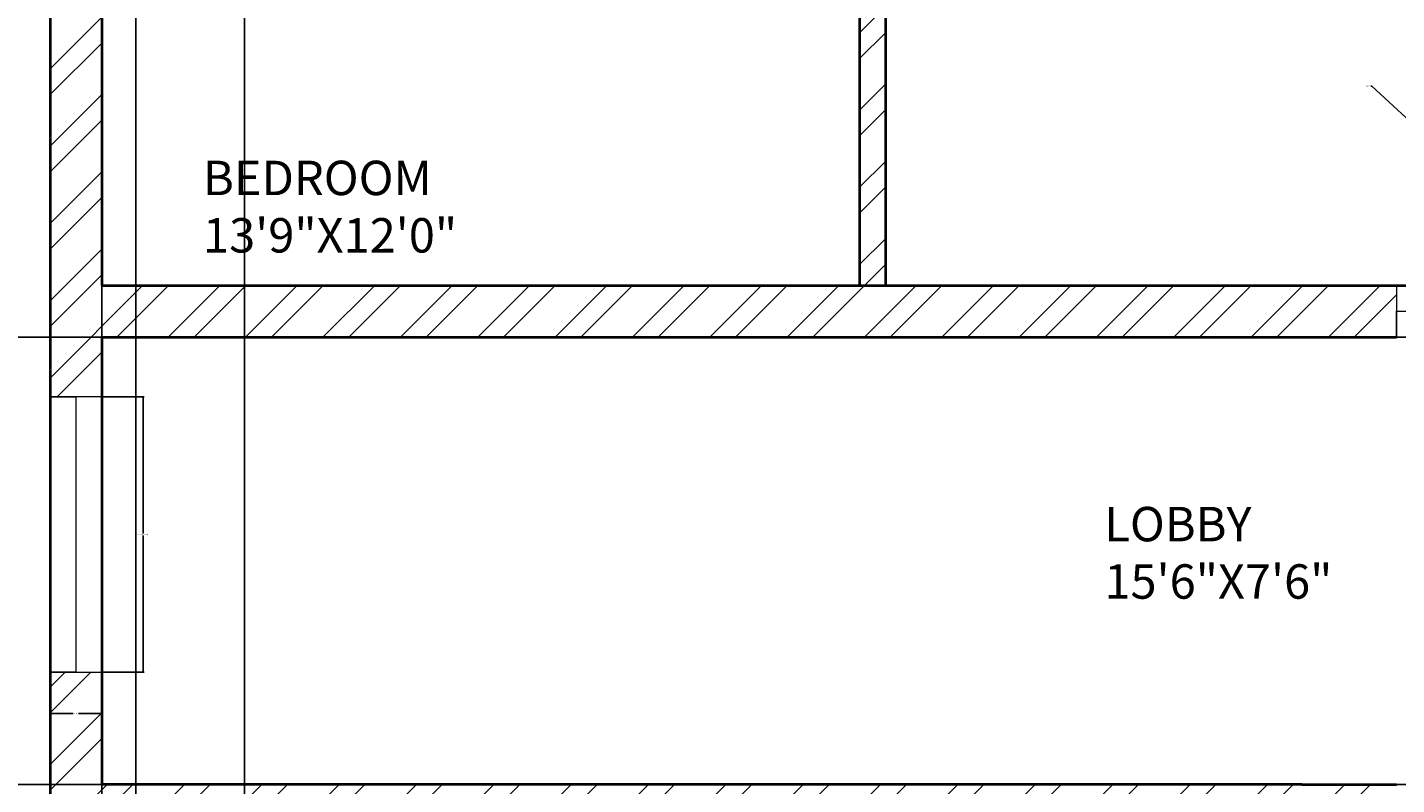
# Model space of a CAD drawing. Units: inches. Extents: x 1355 to 2746, y 1171 to 2751.
# Tile 6 of 24: x 1511 to 1749, y 1686 to 1818. Entities that reach past the tile are written whole.
import ezdxf

# ---------------------------------------------------------------- set-up
doc = ezdxf.new("R2010")
doc.units = ezdxf.units.IN
for name, color, linetype, lineweight in [('A-ANNO-DIMS', 2, 'Continuous', 18), ('A-AREA-IDEN', 7, 'Continuous', 18), ('A-DOOR', 3, 'Continuous', 20), ('A-GLAZ', 4, 'Continuous', 18), ('A-WALL', 7, 'Continuous', 40), ('A-WALL-PATT', 252, 'Continuous', 13)]:
    doc.layers.add(name, color=color, linetype=linetype, lineweight=lineweight)
doc.styles.get("Standard").update_dxf_attribs({"font": 'arial.ttf'})
doc.dimstyles.get("Standard").update_dxf_attribs({"dimtxt": 0.18, "dimasz": 0.18, "dimexe": 0.18, "dimexo": 0.0625, "dimgap": 0.09, "dimtad": 0, "dimtih": 1, "dimtoh": 1, "dimdec": 4, "dimzin": 0, "dimdsep": 46, "dimtxsty": 'Standard', "dimcen": 0.09, "dimadec": 0, "dimazin": 0, "dimtfac": 1, "dimtdec": 4, "dimtofl": 0, "dimtmove": 0, "dimatfit": 3, "dimfxl": 1, "dimtolj": 1, "dimtzin": 0, "dimarcsym": 0})

# ---------------------------------------------------------------- blocks, each defined once
blk = doc.blocks.new('WINDOW-PLAN-48')
for p, q in [((9, 48), (0, 48)), ((0, 48), (4.5, 48)), ((4.5, 48), (4.5, 12)), ((4.5, 12), (4.5, 0)), ((4.5, 0), (0, 0)), ((0, 0), (9, 0))]:
    blk.add_line(p, q)
blk = doc.blocks.new('DOOR-ENTRY-N')
for p, q in [((35.29, 4.5), (35.29, 40.5)), ((0, 9), (0, 0)), ((37.29, 9), (37.29, 0)), ((0, 0), (0, 4.5)), ((0, 4.5), (2, 4.5)), ((37.29, 4.5), (35.29, 4.5)), ((37.29, 0), (37.29, 4.5))]:
    blk.add_line(p, q)
blk.add_arc((38.11, 4.5), 36.11, 94.4716, 180)
blk = doc.blocks.new('*D45')
at = {"layer": 'A-ANNO-DIMS', "color": 0, "lineweight": -2, "transparency": 16777216}
for p, q in [((1523.77, 1753.9), (1531.09, 1753.9)), ((1530.91, 1753.72), (1530.91, 1730.09)), ((1530.91, 1706.08), (1530.91, 1729.72)), ((1523.77, 1705.9), (1531.09, 1705.9))]:
    blk.add_line(p, q, dxfattribs=at)
at = {"layer": 'A-ANNO-DIMS', "color": 0, "transparency": 16777216}
for points in [[(1530.88, 1753.72), (1530.94, 1753.72), (1530.91, 1753.9)], [(1530.88, 1706.08), (1530.94, 1706.08), (1530.91, 1705.9)]]:
    blk.add_solid(points, dxfattribs=at)
at = {"layer": 'Defpoints', "color": 0, "transparency": 16777216}
for p in [(1523.71, 1753.9), (1530.91, 1753.9), (1523.71, 1705.9)]:
    blk.add_point(p, dxfattribs=at)
at = {"layer": 'A-ANNO-DIMS', "color": 0, "transparency": 16777216, "insert": (1530.91, 1729.9), "char_height": 0.18, "attachment_point": 5}
blk.add_mtext('\\A1;WINDOW 48 TYP.', dxfattribs=at)
blk = doc.blocks.new('*D46')
at = {"layer": 'A-ANNO-DIMS', "color": 0, "lineweight": -2, "transparency": 16777216}
for p, q in [((1514.71, 1705.84), (1514.71, 1698.52)), ((1523.71, 1705.84), (1523.71, 1698.52)), ((1514.89, 1698.7), (1518.75, 1698.7)), ((1523.53, 1698.7), (1519.67, 1698.7))]:
    blk.add_line(p, q, dxfattribs=at)
at = {"layer": 'A-ANNO-DIMS', "color": 0, "transparency": 16777216}
for points in [[(1514.89, 1698.73), (1514.89, 1698.67), (1514.71, 1698.7)], [(1523.53, 1698.73), (1523.53, 1698.67), (1523.71, 1698.7)]]:
    blk.add_solid(points, dxfattribs=at)
at = {"layer": 'Defpoints', "color": 0, "transparency": 16777216}
for p in [(1514.71, 1705.9), (1523.71, 1705.9), (1523.71, 1698.7)]:
    blk.add_point(p, dxfattribs=at)
at = {"layer": 'A-ANNO-DIMS', "color": 0, "transparency": 16777216, "insert": (1519.21, 1698.7), "char_height": 0.18, "attachment_point": 5}
blk.add_mtext('\\A1;9 TYP.', dxfattribs=at)
blk = doc.blocks.new('*D96')
at = {"layer": 'A-ANNO-DIMS', "color": 0, "lineweight": -2, "transparency": 16777216}
for p, q in [((1514.65, 2139.3), (1407.53, 2139.3)), ((1407.71, 2139.12), (1407.71, 1725.48)), ((1407.71, 1311.48), (1407.71, 1725.12)), ((1514.65, 1311.3), (1407.53, 1311.3))]:
    blk.add_line(p, q, dxfattribs=at)
at = {"layer": 'A-ANNO-DIMS', "color": 0, "transparency": 16777216}
for points in [[(1407.68, 2139.12), (1407.74, 2139.12), (1407.71, 2139.3)], [(1407.68, 1311.48), (1407.74, 1311.48), (1407.71, 1311.3)]]:
    blk.add_solid(points, dxfattribs=at)
at = {"layer": 'Defpoints', "color": 0, "transparency": 16777216}
for p in [(1407.71, 2139.3), (1514.71, 2139.3), (1514.71, 1311.3)]:
    blk.add_point(p, dxfattribs=at)
at = {"layer": 'A-ANNO-DIMS', "color": 0, "transparency": 16777216, "insert": (1407.71, 1725.3), "char_height": 0.18, "attachment_point": 5}
blk.add_mtext('\\A1;828', dxfattribs=at)
blk = doc.blocks.new('*D102')
at = {"layer": 'A-ANNO-DIMS', "color": 0, "lineweight": -2, "transparency": 16777216}
for p, q in [((2089.33, 1764.3), (1407.53, 1764.3)), ((1407.71, 1764.12), (1407.71, 1725.48)), ((1407.71, 1686.48), (1407.71, 1725.12)), ((2089.33, 1686.3), (1407.53, 1686.3))]:
    blk.add_line(p, q, dxfattribs=at)
at = {"layer": 'A-ANNO-DIMS', "color": 0, "transparency": 16777216}
for points in [[(1407.68, 1764.12), (1407.74, 1764.12), (1407.71, 1764.3)], [(1407.68, 1686.48), (1407.74, 1686.48), (1407.71, 1686.3)]]:
    blk.add_solid(points, dxfattribs=at)
at = {"layer": 'Defpoints', "color": 0, "transparency": 16777216}
for p in [(1407.71, 1764.3), (2089.39, 1764.3), (2089.39, 1686.3)]:
    blk.add_point(p, dxfattribs=at)
at = {"layer": 'A-ANNO-DIMS', "color": 0, "transparency": 16777216, "insert": (1407.71, 1725.3), "char_height": 0.18, "attachment_point": 5}
blk.add_mtext('\\A1;78', dxfattribs=at)
blk = doc.blocks.new('*D103')
at = {"layer": 'A-ANNO-DIMS', "color": 0, "lineweight": -2, "transparency": 16777216}
for p, q in [((2089.33, 1917.3), (1407.53, 1917.3)), ((1407.71, 1917.12), (1407.71, 1840.98)), ((1407.71, 1764.48), (1407.71, 1840.62)), ((2089.33, 1764.3), (1407.53, 1764.3))]:
    blk.add_line(p, q, dxfattribs=at)
at = {"layer": 'A-ANNO-DIMS', "color": 0, "transparency": 16777216}
for points in [[(1407.68, 1917.12), (1407.74, 1917.12), (1407.71, 1917.3)], [(1407.68, 1764.48), (1407.74, 1764.48), (1407.71, 1764.3)]]:
    blk.add_solid(points, dxfattribs=at)
at = {"layer": 'Defpoints', "color": 0, "transparency": 16777216}
for p in [(1407.71, 1917.3), (2089.39, 1917.3), (2089.39, 1764.3)]:
    blk.add_point(p, dxfattribs=at)
at = {"layer": 'A-ANNO-DIMS', "color": 0, "transparency": 16777216, "insert": (1407.71, 1840.8), "char_height": 0.18, "attachment_point": 5}
blk.add_mtext('\\A1;153', dxfattribs=at)
blk = doc.blocks.new('*D107')
at = {"layer": 'A-ANNO-DIMS', "color": 0, "lineweight": -2, "transparency": 16777216}
for p, q in [((2089.33, 1686.3), (1407.53, 1686.3)), ((1407.71, 1686.12), (1407.71, 1622.26)), ((1407.71, 1558.03), (1407.71, 1621.89)), ((2031.09, 1557.85), (1407.53, 1557.85))]:
    blk.add_line(p, q, dxfattribs=at)
at = {"layer": 'A-ANNO-DIMS', "color": 0, "transparency": 16777216}
for points in [[(1407.68, 1686.12), (1407.74, 1686.12), (1407.71, 1686.3)], [(1407.68, 1558.03), (1407.74, 1558.03), (1407.71, 1557.85)]]:
    blk.add_solid(points, dxfattribs=at)
at = {"layer": 'Defpoints', "color": 0, "transparency": 16777216}
for p in [(1407.71, 1686.3), (2089.39, 1686.3), (2031.15, 1557.85)]:
    blk.add_point(p, dxfattribs=at)
at = {"layer": 'A-ANNO-DIMS', "color": 0, "transparency": 16777216, "insert": (1407.71, 1622.07), "char_height": 0.18, "attachment_point": 5}
blk.add_mtext('\\A1;128.46', dxfattribs=at)
blk = doc.blocks.new('*D137')
at = {"layer": 'A-ANNO-DIMS', "color": 0, "lineweight": -2, "transparency": 16777216}
for p, q in [((1523.71, 1921.74), (1523.71, 1171.06)), ((1529.67, 1919.49), (1529.67, 1171.06)), ((1523.89, 1171.24), (1526.36, 1171.24)), ((1529.49, 1171.24), (1527.01, 1171.24))]:
    blk.add_line(p, q, dxfattribs=at)
at = {"layer": 'A-ANNO-DIMS', "color": 0, "transparency": 16777216}
for points in [[(1523.89, 1171.27), (1523.89, 1171.21), (1523.71, 1171.24)], [(1529.49, 1171.27), (1529.49, 1171.21), (1529.67, 1171.24)]]:
    blk.add_solid(points, dxfattribs=at)
at = {"layer": 'Defpoints', "color": 0, "transparency": 16777216}
for p in [(1523.71, 1921.8), (1529.67, 1919.55), (1529.67, 1171.24)]:
    blk.add_point(p, dxfattribs=at)
at = {"layer": 'A-ANNO-DIMS', "color": 0, "transparency": 16777216, "insert": (1526.69, 1171.24), "char_height": 0.18, "attachment_point": 5}
blk.add_mtext('\\A1;5.96', dxfattribs=at)
blk = doc.blocks.new('*D140')
at = {"layer": 'A-ANNO-DIMS', "color": 0, "lineweight": -2, "transparency": 16777216}
for p, q in [((1523.71, 1973.05), (1523.71, 1171.06)), ((1548.6, 1963.94), (1548.6, 1171.06)), ((1523.89, 1171.24), (1535.76, 1171.24)), ((1548.42, 1171.24), (1536.55, 1171.24))]:
    blk.add_line(p, q, dxfattribs=at)
at = {"layer": 'A-ANNO-DIMS', "color": 0, "transparency": 16777216}
for points in [[(1523.89, 1171.27), (1523.89, 1171.21), (1523.71, 1171.24)], [(1548.42, 1171.27), (1548.42, 1171.21), (1548.6, 1171.24)]]:
    blk.add_solid(points, dxfattribs=at)
at = {"layer": 'Defpoints', "color": 0, "transparency": 16777216}
for p in [(1523.71, 1973.11), (1548.6, 1964.01), (1548.6, 1171.24)]:
    blk.add_point(p, dxfattribs=at)
at = {"layer": 'A-ANNO-DIMS', "color": 0, "transparency": 16777216, "insert": (1536.15, 1171.24), "char_height": 0.18, "attachment_point": 5}
blk.add_mtext('\\A1;24.89', dxfattribs=at)
blk = doc.blocks.new('*D154')
at = {"layer": 'A-ANNO-DIMS', "color": 0, "lineweight": -2, "transparency": 16777216}
for p, q in [((1744.73, 1808.03), (1744.91, 1808.03)), ((1744.91, 1808.03), (1760.69, 1793.44)), ((1787.24, 1768.8), (1787.42, 1768.8)), ((1787.33, 1768.71), (1787.33, 1768.89))]:
    blk.add_line(p, q, dxfattribs=at)
at = {"layer": 'A-ANNO-DIMS', "color": 0, "transparency": 16777216}
blk.add_solid([(1760.71, 1793.46), (1760.67, 1793.42), (1760.82, 1793.32)], dxfattribs=at)
at = {"layer": 'Defpoints', "color": 0, "transparency": 16777216}
for p in [(1760.82, 1793.32), (1787.33, 1768.8)]:
    blk.add_point(p, dxfattribs=at)
at = {"layer": 'A-ANNO-DIMS', "color": 0, "transparency": 16777216, "insert": (1744.27, 1808.03), "char_height": 0.18, "attachment_point": 5}
blk.add_mtext('\\A1;R36.11', dxfattribs=at)

msp = doc.modelspace()

# ---------------------------------------------------------------- hatches: boundary and pattern name
at = {"layer": 'A-WALL-PATT'}
h = msp.add_hatch(dxfattribs=at)
h.set_pattern_fill('ANSI32', color=256)
h.paths.add_polyline_path([(1660.2083, 2139.3018), (1614.5977, 2139.3018), (1614.5977, 2130.3018), (1655.7083, 2130.3018), (1655.7083, 1981.8018), (1660.2083, 1981.8018), (1660.2083, 2090.7225), (1692.5832, 2090.7225), (1692.5832, 2095.2225), (1660.2083, 2095.2225)])
h.paths.add_polyline_path([(1523.7083, 2130.3018), (1554.5977, 2130.3018), (1554.5977, 2134.8018), (1554.5977, 2139.3018), (1514.7083, 2139.3018), (1514.7083, 2071.8385), (1523.7083, 2071.8385)])
h.paths.add_polyline_path([(1940.7083, 2139.3018), (1883.7928, 2139.3018), (1883.7928, 2130.3018), (1931.7083, 2130.3018), (1931.7083, 2098.3333), (1940.7083, 2098.3333)])
h.paths.add_polyline_path([(1799.7083, 2130.3018), (1823.7928, 2130.3018), (1823.7928, 2134.8018), (1823.7928, 2139.3018), (1795.2083, 2139.3018), (1795.2083, 2130.3018), (1795.2083, 2095.2225), (1759.2134, 2095.2225), (1759.2134, 2090.7225), (1795.2083, 2090.7225), (1795.2083, 1981.8018), (1799.7083, 1981.8018), (1799.7083, 1986.3018)])
h.paths.add_polyline_path([(1940.7083, 2038.3333), (1931.7083, 2038.3333), (1931.7083, 1986.3018), (1832.7083, 1986.3018), (1832.7083, 1947.1338), (1837.2083, 1947.1338), (1837.2083, 1981.8018), (1931.7083, 1981.8018), (1931.7083, 1967.1939), (1940.7083, 1967.1939)])
h.paths.add_polyline_path([(1940.7083, 1943.1939), (1931.7083, 1943.1939), (1931.7083, 1921.8018), (1837.2083, 1921.8018), (1837.2083, 1926.0511), (1832.7083, 1926.0511), (1832.7083, 1917.3018), (1931.7083, 1917.3018), (1931.7083, 1908.3321), (1940.7083, 1908.3321)])
h.paths.add_polyline_path([(1940.7083, 1884.3321), (1931.7083, 1884.3321), (1931.7083, 1869.3018), (1899.4583, 1869.3018), (1899.4583, 1864.8018), (1931.7083, 1864.8018), (1931.7083, 1773.3018), (1786.5143, 1773.3018), (1786.5143, 1764.3018), (1844.7083, 1764.3018), (1844.7083, 1748.9343), (1853.7083, 1748.9343), (1853.7083, 1764.3018), (1931.7083, 1764.3018), (1931.7083, 1652.9424), (1940.7083, 1652.9424)])
h.paths.add_polyline_path([(1799.7083, 1864.8018), (1806.0522, 1864.8018), (1806.0522, 1867.0518), (1806.0522, 1869.3018), (1799.7083, 1869.3018), (1799.7083, 1917.3018), (1799.7083, 1921.8018), (1795.2083, 1921.8018), (1795.2083, 1773.3018), (1799.7083, 1773.3018)])
h.paths.add_polyline_path([(1872.8988, 1867.0518), (1872.8988, 1869.3018), (1867.2083, 1869.3018), (1867.2083, 1917.3018), (1862.7083, 1917.3018), (1862.7083, 1869.3018), (1836.9546, 1869.3018), (1836.9546, 1864.8018), (1862.7083, 1864.8018), (1872.8988, 1864.8018)])
h.paths.add_polyline_path([(1749.2197, 1773.3018), (1655.7083, 1773.3018), (1523.7083, 1773.3018), (1523.7083, 1828.4963), (1514.7083, 1828.4963), (1514.7083, 1753.9033), (1519.2083, 1753.9033), (1523.7083, 1753.9033), (1523.7083, 1764.3018), (1655.7083, 1764.3018), (1749.2197, 1764.3018), (1749.2197, 1768.8018)])
h.paths.add_polyline_path([(1660.2083, 1921.8018), (1655.7083, 1921.8018), (1655.7083, 1917.3018), (1655.7083, 1773.3018), (1660.2083, 1773.3018)])
h.paths.add_polyline_path([(1523.7083, 2011.8385), (1514.7083, 2011.8385), (1514.7083, 1973.114), (1519.2083, 1973.114), (1523.7083, 1973.114), (1523.7083, 1976.8227), (1523.7083, 1981.8018), (1618.2083, 1981.8018), (1618.2083, 1921.8018), (1553.707, 1921.8018), (1553.707, 1917.3018), (1622.7083, 1917.3018), (1622.7083, 1919.5518), (1622.7083, 1921.8018), (1622.7083, 1986.3018), (1523.7083, 1986.3018)])
h.paths.add_polyline_path([(1529.6686, 1919.5518), (1529.6686, 1921.8018), (1523.7083, 1921.8018), (1523.7083, 1949.114), (1514.7083, 1949.114), (1514.7083, 1888.4963), (1523.7083, 1888.4963), (1523.7083, 1917.3018), (1529.6686, 1917.3018)])
h.paths.add_polyline_path([(1538.9419, 1775.643), (1585.5504, 1775.643), (1585.5504, 1798.0318), (1538.9419, 1798.0318)], flags=25)
h.paths.add_polyline_path([(1696.7097, 1497.3356), (1769.5651, 1497.3356), (1769.5651, 1523.4559), (1696.7097, 1523.4559)], flags=9)
h.paths.add_polyline_path([(1629.1643, 1230.5133), (1877.0879, 1230.5133), (1877.0879, 1267.606), (1629.1643, 1267.606)], flags=9)
h.paths.add_polyline_path([(2533.4462, 2215.4033), (2579.9292, 2215.4033), (2579.9292, 2231.889), (2533.4462, 2231.889)], flags=9)
h.paths.add_polyline_path([(2540.822, 2515.6945), (2594.2245, 2515.6945), (2594.2245, 2545.5463), (2540.822, 2545.5463)], flags=9)
h.paths.add_polyline_path([(2535.9857, 2588.2819), (2582.4687, 2588.2819), (2582.4687, 2604.7675), (2535.9857, 2604.7675)], flags=9)
h.paths.add_polyline_path([(2537.1627, 2617.1172), (2649.1245, 2617.1172), (2649.1245, 2633.6029), (2537.1627, 2633.6029)], flags=9)
h.paths.add_polyline_path([(2218.0051, 2168.228), (2363.9573, 2168.228), (2363.9573, 2205.3208), (2218.0051, 2205.3208)], flags=9)
h.paths.add_polyline_path([(1650.2156, 2165.3631), (1800.3547, 2165.3631), (1800.3547, 2202.4559), (1650.2156, 2202.4559)], flags=9)
h.paths.add_polyline_path([(2553.9592, 1610.7663), (2588.4203, 1610.7663), (2588.4203, 1660.2233), (2553.9592, 1660.2233)], flags=9)
h.paths.add_polyline_path([(1549.0868, 1648.2033), (1595.6952, 1648.2033), (1595.6952, 1670.5921), (1549.0868, 1670.5921)], flags=9)
h.paths.add_polyline_path([(1546.9525, 1502.0931), (1583.3413, 1502.0931), (1583.3413, 1524.4819), (1546.9525, 1524.4819)], flags=9)
h.paths.add_polyline_path([(1540.7704, 1433.4431), (1587.3788, 1433.4431), (1587.3788, 1455.8319), (1540.7704, 1455.8319)], flags=9)
h.paths.add_polyline_path([(1683.6524, 1321.5269), (1760.6169, 1321.5269), (1760.6169, 1333.8911), (1683.6524, 1333.8911)], flags=9)
h.paths.add_polyline_path([(1832.0485, 1356.0874), (1873.0989, 1356.0874), (1873.0989, 1378.4762), (1832.0485, 1378.4762)], flags=9)
h.paths.add_polyline_path([(1877.9694, 1431.2138), (1926.3827, 1431.2138), (1926.3827, 1453.578), (1877.9694, 1453.578)], flags=9)
h.paths.add_polyline_path([(1847.3106, 1499.8371), (1883.6994, 1499.8371), (1883.6994, 1522.2259), (1847.3106, 1522.2259)], flags=9)
h.paths.add_polyline_path([(1813.7015, 1640.7287), (1860.3099, 1640.7287), (1860.3099, 1663.1175), (1813.7015, 1663.1175)], flags=9)
h.paths.add_polyline_path([(1876.2576, 1710.2471), (1912.9452, 1710.2471), (1912.9452, 1732.6359), (1876.2576, 1732.6359)], flags=25)
h.paths.add_polyline_path([(1695.9163, 1715.3064), (1736.9668, 1715.3064), (1736.9668, 1737.6952), (1695.9163, 1737.6952)], flags=9)
h.paths.add_polyline_path([(1881.8583, 1888.9094), (1930.2717, 1888.9094), (1930.2717, 1911.2737), (1881.8583, 1911.2737)], flags=9)
h.paths.add_polyline_path([(1823.9298, 1798.6431), (1864.9803, 1798.6431), (1864.9803, 1821.0319), (1823.9298, 1821.0319)], flags=25)
h.paths.add_polyline_path([(1845.6062, 1948.1408), (1881.995, 1948.1408), (1881.995, 1970.5296), (1845.6062, 1970.5296)], flags=25)
h.paths.add_polyline_path([(1849.027, 1991.5151), (1895.6355, 1991.5151), (1895.6355, 2013.9039), (1849.027, 2013.9039)], flags=25)
h.paths.add_polyline_path([(1684.9725, 2113.8416), (1764.2658, 2113.8416), (1764.2658, 2126.2058), (1684.9725, 2126.2058)], flags=9)
h.paths.add_polyline_path([(1688.6193, 1913.0676), (1776.2005, 1913.0676), (1776.2005, 1935.4564), (1688.6193, 1935.4564)], flags=9)
h.paths.add_polyline_path([(1571.4689, 1930.9816), (1607.8577, 1930.9816), (1607.8577, 1953.3704), (1571.4689, 1953.3704)], flags=25)
h.paths.add_polyline_path([(1535.3581, 1998.3125), (1581.9665, 1998.3125), (1581.9665, 2020.7014), (1535.3581, 2020.7014)], flags=9)
h = msp.add_hatch(dxfattribs=at)
h.set_pattern_fill('ANSI32', color=256)
h.paths.add_polyline_path([(1749.2197, 1686.3018), (1732.6892, 1686.3018), (1523.7083, 1686.3018), (1523.7083, 1705.9033), (1514.7083, 1705.9033), (1514.7083, 1647.8732), (1519.2083, 1647.8732), (1523.7083, 1647.8732), (1523.7083, 1677.3018), (1655.7083, 1677.3018), (1655.7083, 1528.8018), (1660.2083, 1528.8018), (1660.2083, 1677.3018), (1732.6892, 1677.3018), (1749.2197, 1677.3018)])
h.paths.add_polyline_path([(1931.7083, 1686.3018), (1853.7083, 1686.3018), (1853.7083, 1703.5696), (1844.7083, 1703.5696), (1844.7083, 1686.3018), (1788.0274, 1686.3018), (1788.0274, 1677.3018), (1795.2083, 1677.3018), (1795.2083, 1528.8018), (1799.7083, 1528.8018), (1799.7083, 1677.3018), (1844.7083, 1677.3018), (1931.7083, 1677.3018)])
h.paths.add_polyline_path([(1931.7083, 1533.3018), (1844.7083, 1533.3018), (1832.7083, 1533.3018), (1832.7083, 1531.0518), (1832.7083, 1528.8018), (1832.7083, 1495.7519), (1837.2083, 1495.7519), (1837.2083, 1528.8018), (1931.7083, 1528.8018)])
h.paths.add_polyline_path([(1940.7083, 1592.9424), (1931.7083, 1592.9424), (1931.7083, 1506.7845), (1940.7083, 1506.7845)])
h.paths.add_polyline_path([(1940.7083, 1482.7845), (1936.2083, 1482.7845), (1931.7083, 1482.7845), (1931.7083, 1320.3018), (1880.7083, 1320.3018), (1880.7083, 1311.3018), (1940.7083, 1311.3018)])
h.paths.add_polyline_path([(1931.7083, 1468.8018), (1844.7083, 1468.8018), (1837.2083, 1468.8018), (1837.2083, 1474.34), (1832.7083, 1474.34), (1832.7083, 1468.8018), (1832.7083, 1464.3018), (1844.7083, 1464.3018), (1931.7083, 1464.3018)])
h.paths.add_polyline_path([(1863.8571, 1464.3018), (1859.3571, 1464.3018), (1859.3571, 1404.1662), (1838.1542, 1404.1662), (1838.1542, 1399.8018), (1869.4185, 1399.8018), (1869.4185, 1402.0518), (1869.4185, 1404.3018), (1863.8571, 1404.3018)])
h.paths.add_polyline_path([(1799.7083, 1399.6662), (1805.4082, 1399.6662), (1805.4082, 1401.9162), (1805.4082, 1404.1662), (1799.7083, 1404.1662), (1799.7083, 1464.3018), (1799.7083, 1468.8018), (1795.2083, 1468.8018), (1795.2083, 1356.2098), (1761.2597, 1356.2098), (1761.2597, 1351.7098), (1795.2083, 1351.7098), (1795.2083, 1320.3018), (1795.2083, 1311.3018), (1844.7083, 1311.3018), (1844.7083, 1315.8018), (1844.7083, 1320.3018), (1799.7083, 1320.3018)])
h.paths.add_polyline_path([(1692.9218, 1356.2098), (1660.2083, 1356.2098), (1660.2083, 1430.786), (1657.9583, 1430.786), (1655.7083, 1430.786), (1655.7083, 1320.3018), (1611.934, 1320.3018), (1611.934, 1311.3018), (1660.2083, 1311.3018), (1660.2083, 1351.7098), (1692.9218, 1351.7098)])
h.paths.add_polyline_path([(1523.7083, 1372.653), (1514.7083, 1372.653), (1514.7083, 1311.3018), (1551.934, 1311.3018), (1551.934, 1315.8018), (1551.934, 1320.3018), (1523.7083, 1320.3018)])
h.paths.add_polyline_path([(1523.7083, 1490.9023), (1514.7083, 1490.9023), (1514.7083, 1432.653), (1519.2083, 1432.653), (1523.7083, 1432.653)])
h.paths.add_polyline_path([(1660.2083, 1468.8018), (1622.7083, 1468.8018), (1622.7083, 1473.1566), (1618.2083, 1473.1566), (1618.2083, 1468.8018), (1523.7083, 1468.8018), (1523.7083, 1464.3018), (1655.7083, 1464.3018), (1655.7083, 1460.5634), (1660.2083, 1460.5634)])
h.paths.add_polyline_path([(1523.7083, 1587.8732), (1514.7083, 1587.8732), (1514.7083, 1514.9023), (1519.2083, 1514.9023), (1523.7083, 1514.9023)])
h.paths.add_polyline_path([(1622.7083, 1533.3018), (1523.7083, 1533.3018), (1523.7083, 1528.8018), (1618.2083, 1528.8018), (1618.2083, 1494.4205), (1622.7083, 1494.4205), (1622.7083, 1528.8018)])
h.paths.add_polyline_path([(1696.7097, 1497.3356), (1769.5651, 1497.3356), (1769.5651, 1523.4559), (1696.7097, 1523.4559)], flags=9)
h.paths.add_polyline_path([(1629.1643, 1230.5133), (1877.0879, 1230.5133), (1877.0879, 1267.606), (1629.1643, 1267.606)], flags=9)
h.paths.add_polyline_path([(2533.4462, 2215.4033), (2579.9292, 2215.4033), (2579.9292, 2231.889), (2533.4462, 2231.889)], flags=9)
h.paths.add_polyline_path([(2540.822, 2515.6945), (2594.2245, 2515.6945), (2594.2245, 2545.5463), (2540.822, 2545.5463)], flags=9)
h.paths.add_polyline_path([(2535.9857, 2588.2819), (2582.4687, 2588.2819), (2582.4687, 2604.7675), (2535.9857, 2604.7675)], flags=9)
h.paths.add_polyline_path([(2537.1627, 2617.1172), (2649.1245, 2617.1172), (2649.1245, 2633.6029), (2537.1627, 2633.6029)], flags=9)
h.paths.add_polyline_path([(2218.0051, 2168.228), (2363.9573, 2168.228), (2363.9573, 2205.3208), (2218.0051, 2205.3208)], flags=9)
h.paths.add_polyline_path([(1650.2156, 2165.3631), (1800.3547, 2165.3631), (1800.3547, 2202.4559), (1650.2156, 2202.4559)], flags=9)
h.paths.add_polyline_path([(2553.9592, 1610.7663), (2588.4203, 1610.7663), (2588.4203, 1660.2233), (2553.9592, 1660.2233)], flags=9)
h.paths.add_polyline_path([(1549.0868, 1648.2033), (1595.6952, 1648.2033), (1595.6952, 1670.5921), (1549.0868, 1670.5921)], flags=25)
h.paths.add_polyline_path([(1546.9525, 1502.0931), (1583.3413, 1502.0931), (1583.3413, 1524.4819), (1546.9525, 1524.4819)], flags=25)
h.paths.add_polyline_path([(1540.7704, 1433.4431), (1587.3788, 1433.4431), (1587.3788, 1455.8319), (1540.7704, 1455.8319)], flags=9)
h.paths.add_polyline_path([(1683.6524, 1321.5269), (1760.6169, 1321.5269), (1760.6169, 1333.8911), (1683.6524, 1333.8911)], flags=9)
h.paths.add_polyline_path([(1832.0485, 1356.0874), (1873.0989, 1356.0874), (1873.0989, 1378.4762), (1832.0485, 1378.4762)], flags=9)
h.paths.add_polyline_path([(1877.9694, 1431.2138), (1926.3827, 1431.2138), (1926.3827, 1453.578), (1877.9694, 1453.578)], flags=9)
h.paths.add_polyline_path([(1847.3106, 1499.8371), (1883.6994, 1499.8371), (1883.6994, 1522.2259), (1847.3106, 1522.2259)], flags=25)
h.paths.add_polyline_path([(1813.7015, 1640.7287), (1860.3099, 1640.7287), (1860.3099, 1663.1175), (1813.7015, 1663.1175)], flags=25)
h.paths.add_polyline_path([(1876.2576, 1710.2471), (1912.9452, 1710.2471), (1912.9452, 1732.6359), (1876.2576, 1732.6359)], flags=9)
h.paths.add_polyline_path([(1695.9163, 1715.3064), (1736.9668, 1715.3064), (1736.9668, 1737.6952), (1695.9163, 1737.6952)], flags=9)
h.paths.add_polyline_path([(1881.8583, 1888.9094), (1930.2717, 1888.9094), (1930.2717, 1911.2737), (1881.8583, 1911.2737)], flags=9)
h.paths.add_polyline_path([(1823.9298, 1798.6431), (1864.9803, 1798.6431), (1864.9803, 1821.0319), (1823.9298, 1821.0319)], flags=9)
h.paths.add_polyline_path([(1845.6062, 1948.1408), (1881.995, 1948.1408), (1881.995, 1970.5296), (1845.6062, 1970.5296)], flags=9)
h.paths.add_polyline_path([(1849.027, 1991.5151), (1895.6355, 1991.5151), (1895.6355, 2013.9039), (1849.027, 2013.9039)], flags=9)
h.paths.add_polyline_path([(1684.9725, 2113.8416), (1764.2658, 2113.8416), (1764.2658, 2126.2058), (1684.9725, 2126.2058)], flags=9)
h.paths.add_polyline_path([(1688.6193, 1913.0676), (1776.2005, 1913.0676), (1776.2005, 1935.4564), (1688.6193, 1935.4564)], flags=9)
h.paths.add_polyline_path([(1538.9419, 1775.643), (1585.5504, 1775.643), (1585.5504, 1798.0318), (1538.9419, 1798.0318)], flags=9)
h.paths.add_polyline_path([(1571.4689, 1930.9816), (1607.8577, 1930.9816), (1607.8577, 1953.3704), (1571.4689, 1953.3704)], flags=9)
h.paths.add_polyline_path([(1535.3581, 1998.3125), (1581.9665, 1998.3125), (1581.9665, 2020.7014), (1535.3581, 2020.7014)], flags=9)

# ---------------------------------------------------------------- linework, layer by layer
at = {"layer": 'A-WALL'}
for p, q in [((1514.7083, 2139.3018), (1514.7083, 1311.3018)), ((1660.2083, 1921.8018), (1660.2083, 1773.3018)), ((1523.7083, 1917.3018), (1523.7083, 1773.3018)), ((1655.7083, 1917.3018), (1655.7083, 1773.3018)), ((1523.7083, 1773.3018), (1655.7083, 1773.3018)), ((1655.7083, 1773.3018), (1751.5012, 1773.3018)), ((1523.7083, 1764.3018), (1655.7083, 1764.3018)), ((1523.7083, 1764.3018), (1523.7083, 1686.3018)), ((1655.7083, 1764.3018), (1749.2197, 1764.3018)), ((1732.6892, 1686.3018), (1523.7083, 1686.3018)), ((1732.6892, 1686.3018), (1749.2197, 1686.3018))]:
    msp.add_line(p, q, dxfattribs=at)

# ---------------------------------------------------------------- block references
at = {"layer": 'A-DOOR'}
msp.add_blockref('DOOR-ENTRY-N', (1749.22, 1764.302), dxfattribs=at)
at = {"layer": 'A-GLAZ'}
msp.add_blockref('WINDOW-PLAN-48', (1514.708, 1705.903), dxfattribs=at)

# ---------------------------------------------------------------- texts
at = {"layer": 'A-AREA-IDEN', "char_height": 6, "attachment_point": 1}
for s, width, insert in [('BEDROOM\\P13\'9"X12\'0"', 162.009589, (1541.3546, 1795.0502)), ('LOBBY\\P15\'6"X7\'6" ', 102.024076, (1698.329, 1734.7136))]:
    msp.add_mtext_dynamic_manual_height_columns(s, width=width, gutter_width=12.5, heights=[0], dxfattribs=dict(at, insert=insert))

# ---------------------------------------------------------------- dimensions: what is measured, and where the dimension line sits
at = {"layer": 'A-ANNO-DIMS'}
for base, p1, p2, override, picture, middle in [((1407.7083, 2139.3018), (1514.7083, 1311.3018), (1514.7083, 2139.3018), {"dimdec": 0, "dimlfac": 1, "dimrnd": 0, "dimzin": 0, "dimdsep": 46, "dimlunit": 2}, '*D96', (1407.7083, 1725.3018)), ((1407.7083, 1917.3018), (2089.3909, 1764.3018), (2089.3909, 1917.3018), {"dimdec": 0, "dimlfac": 1, "dimrnd": 0, "dimzin": 0, "dimdsep": 46, "dimlunit": 2}, '*D103', (1407.7083, 1840.8018)), ((1407.7083, 1764.3018), (2089.3909, 1686.3018), (2089.3909, 1764.3018), {"dimdec": 0, "dimlfac": 1, "dimrnd": 0, "dimzin": 0, "dimdsep": 46, "dimlunit": 2}, '*D102', (1407.7083, 1725.3018)), ((1407.7083, 1686.3018), (2031.1535, 1557.845), (2089.3909, 1686.3018), {"dimdec": 2, "dimlfac": 1, "dimrnd": 0, "dimzin": 0, "dimdsep": 46, "dimlunit": 2}, '*D107', (1407.7083, 1622.0734))]:
    dim = msp.add_linear_dim(base=base, p1=p1, p2=p2, angle=90, dimstyle='Standard', override=override, dxfattribs=at)
    dim.commit()
    dim.dimension.update_dxf_attribs({"geometry": picture, "text_midpoint": middle})
for base, p1, p2, picture, middle in [((1548.5973, 1171.2388), (1523.7077, 1973.1139), (1548.5973, 1964.0069), '*D140', (1536.1525, 1171.2388)), ((1529.6686, 1171.2388), (1523.7083, 1921.8018), (1529.6686, 1919.5518), '*D137', (1526.6885, 1171.2388))]:
    dim = msp.add_linear_dim(base=base, p1=p1, p2=p2, dimstyle='Standard', override={"dimdec": 2, "dimlfac": 1, "dimrnd": 0, "dimzin": 0, "dimdsep": 46, "dimlunit": 2}, dxfattribs=at)
    dim.commit()
    dim.dimension.update_dxf_attribs({"geometry": picture, "text_midpoint": middle})
dim = msp.add_radius_dim(center=(1787.3297, 1768.8018), mpoint=(1760.8193, 1793.3197), dimstyle='Standard', override={"dimdec": 2, "dimlfac": 1, "dimrnd": 0, "dimzin": 0, "dimdsep": 46, "dimlunit": 2}, dxfattribs=at)
dim.commit()
dim.dimension.update_dxf_attribs({"geometry": '*D154', "text_midpoint": (1744.2706, 1808.0305), "dimtype": 164})
dim = msp.add_linear_dim(base=(1530.9083, 1753.9033), p1=(1523.7083, 1705.9033), p2=(1523.7083, 1753.9033), angle=90, text='WINDOW <> TYP.', dimstyle='Standard', override={"dimdec": 0, "dimlfac": 1, "dimrnd": 0, "dimzin": 0, "dimdsep": 46, "dimlunit": 2}, dxfattribs=at)
dim.commit()
dim.dimension.update_dxf_attribs({"geometry": '*D45', "text_midpoint": (1530.9083, 1729.9033)})
dim = msp.add_linear_dim(base=(1523.7083, 1698.7033), p1=(1514.7083, 1705.9033), p2=(1523.7083, 1705.9033), text='<> TYP.', dimstyle='Standard', override={"dimdec": 0, "dimlfac": 1, "dimrnd": 0, "dimzin": 0, "dimdsep": 46, "dimlunit": 2}, dxfattribs=at)
dim.commit()
dim.dimension.update_dxf_attribs({"geometry": '*D46', "text_midpoint": (1519.2083, 1698.7033)})

doc.saveas('drawing.dxf')
